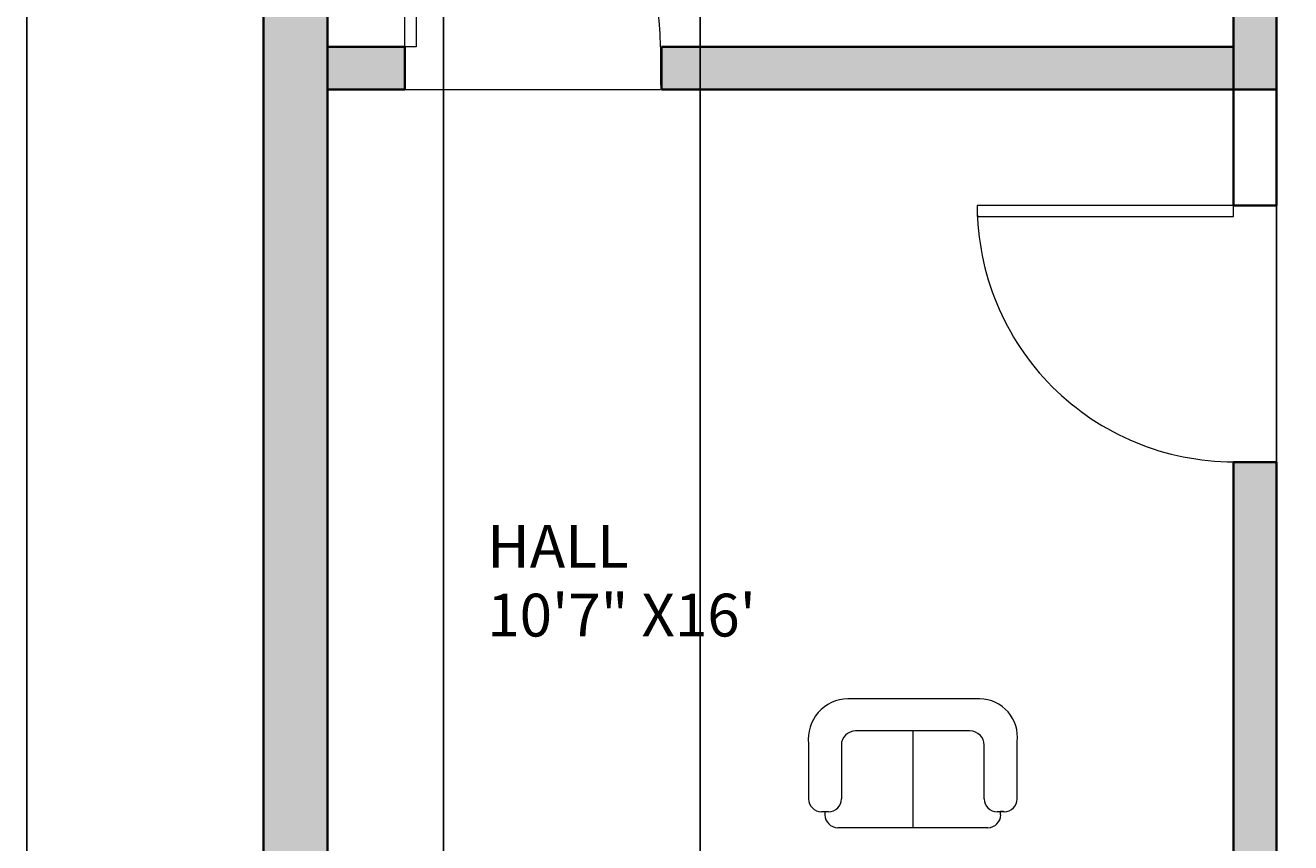
# Model space of a CAD drawing. Units: inches. Extents: x 2070 to 4408, y 1595 to 4269.
# Tile 3 of 20: x 2070 to 2247, y 1835 to 1949. Entities that reach past the tile are written whole.
import ezdxf

# ---------------------------------------------------------------- set-up
doc = ezdxf.new("R2010")
doc.units = ezdxf.units.IN
for name, color, linetype, lineweight in [('A-ANNO-DIMS', 2, 'Continuous', 18), ('A-AREA-IDEN', 7, 'Continuous', 18), ('A-DOOR', 4, 'Continuous', 18), ('A-FURN', 8, 'Continuous', 18), ('A-WALL', 7, 'Continuous', 35)]:
    doc.layers.add(name, color=color, linetype=linetype, lineweight=lineweight)
doc.layers.add('A-WALL-PATT', color=18, linetype='Continuous', lineweight=13, true_color=0x000000)
doc.styles.get("Standard").update_dxf_attribs({"font": 'arial.ttf'})
doc.dimstyles.get("Standard").update_dxf_attribs({"dimtxt": 0.18, "dimasz": 0.18, "dimexe": 0.18, "dimexo": 0.0625, "dimgap": 0.09, "dimtad": 0, "dimtih": 1, "dimtoh": 1, "dimdec": 4, "dimzin": 0, "dimdsep": 46, "dimtxsty": 'Standard', "dimcen": 0.09, "dimadec": 0, "dimazin": 0, "dimtfac": 1, "dimtdec": 4, "dimtofl": 0, "dimtmove": 0, "dimatfit": 3, "dimfxl": 1, "dimtolj": 1, "dimtzin": 0, "dimarcsym": 0})

# ---------------------------------------------------------------- blocks, each defined once
blk = doc.blocks.new('*U4')
for p, q in [((0, 0), (0, -6)), ((40, 0), (40, -6))]:
    blk.add_line(p, q)
blk.add_lwpolyline([(0, 0), (0, 40), (1.75, 40), (1.75, 0)], close=True)
blk.add_arc((0, 0), 40, 0, 90)
blk = doc.blocks.new('*U3')
for p, q in [((0, 0), (0, 6)), ((40, 0), (40, 6))]:
    blk.add_line(p, q)
blk.add_lwpolyline([(0, 0), (0, -40), (1.75, -40), (1.75, 0)], close=True)
blk.add_arc((0, 0), 40, 270, 0)
blk = doc.blocks.new('A$C6D011943')
for p, q in [((1.448, 1.089), (0.332, 1.089)), ((1.364, 0.818), (0.398, 0.818)), ((0.881, 0.818), (0.881, 0)), ((0, 0.709), (0, 0.247)), ((0.278, 0.697), (0.278, 0.244)), ((1.485, 0.244), (1.485, 0.697)), ((1.762, 0.247), (1.762, 0.727)), ((0.109, 0.136), (0.169, 0.136)), ((0.139, 0.109), (0.139, 0.136)), ((1.593, 0.136), (1.654, 0.136)), ((1.648, 0.136), (1.623, 0.136)), ((1.623, 0.109), (1.623, 0.136)), ((1.515, 0), (0.247, 0))]:
    blk.add_line(p, q)
for centre, radius, start, end in [((0.339, 0.748), 0.342, 91.2564, 186.501), ((1.441, 0.766), 0.324, 353.159, 88.6697), ((0.398, 0.697), 0.121, 90, 180), ((1.364, 0.697), 0.121, 0, 90), ((0.109, 0.244), 0.109, 180, 270), ((0.169, 0.244), 0.109, 270, 0), ((1.593, 0.244), 0.109, 180, 270), ((1.654, 0.244), 0.109, 270, 0), ((0.247, 0.109), 0.109, 180, 270), ((1.515, 0.109), 0.109, 270, 0)]:
    blk.add_arc(centre, radius, start, end)
blk = doc.blocks.new('*D24')
at = {"layer": 'A-ANNO-DIMS', "color": 0, "lineweight": -2, "transparency": 16777216}
for p, q in [((2103.13, 2291.4), (2069.84, 2291.4)), ((2070.02, 2291.22), (2070.02, 1960.08)), ((2070.02, 1628.58), (2070.02, 1959.72)), ((2336.13, 1628.4), (2069.84, 1628.4))]:
    blk.add_line(p, q, dxfattribs=at)
at = {"layer": 'A-ANNO-DIMS', "color": 0, "transparency": 16777216}
for points in [[(2069.99, 2291.22), (2070.05, 2291.22), (2070.02, 2291.4)], [(2069.99, 1628.58), (2070.05, 1628.58), (2070.02, 1628.4)]]:
    blk.add_solid(points, dxfattribs=at)
at = {"layer": 'Defpoints', "color": 0, "transparency": 16777216}
for p in [(2070.02, 2291.4), (2103.2, 2291.4), (2336.2, 1628.4)]:
    blk.add_point(p, dxfattribs=at)
at = {"layer": 'A-ANNO-DIMS', "color": 0, "transparency": 16777216, "insert": (2070.02, 1959.9), "char_height": 0.18, "attachment_point": 5}
blk.add_mtext('\\A1;663', dxfattribs=at)
blk = doc.blocks.new('*D29')
at = {"layer": 'A-ANNO-DIMS', "color": 0, "lineweight": -2, "transparency": 16777216}
for p, q in [((2128.44, 2150.34), (2128.44, 1595.04)), ((2164.44, 2150.34), (2164.44, 1595.04)), ((2128.62, 1595.22), (2146.22, 1595.22)), ((2164.26, 1595.22), (2146.65, 1595.22))]:
    blk.add_line(p, q, dxfattribs=at)
at = {"layer": 'A-ANNO-DIMS', "color": 0, "transparency": 16777216}
for points in [[(2128.62, 1595.25), (2128.62, 1595.19), (2128.44, 1595.22)], [(2164.26, 1595.25), (2164.26, 1595.19), (2164.44, 1595.22)]]:
    blk.add_solid(points, dxfattribs=at)
at = {"layer": 'Defpoints', "color": 0, "transparency": 16777216}
for p in [(2128.44, 2150.4), (2164.44, 2150.4), (2164.44, 1595.22)]:
    blk.add_point(p, dxfattribs=at)
at = {"layer": 'A-ANNO-DIMS', "color": 0, "transparency": 16777216, "insert": (2146.44, 1595.22), "char_height": 0.18, "attachment_point": 5}
blk.add_mtext('\\A1;36', dxfattribs=at)
blk = doc.blocks.new('*D32')
at = {"layer": 'A-ANNO-DIMS', "color": 0, "lineweight": -2, "transparency": 16777216}
for p, q in [((2245.2, 2230.58), (2245.2, 1595.04)), ((2340.2, 2230.58), (2340.2, 1595.04)), ((2245.38, 1595.22), (2292.48, 1595.22)), ((2340.02, 1595.22), (2292.92, 1595.22))]:
    blk.add_line(p, q, dxfattribs=at)
at = {"layer": 'A-ANNO-DIMS', "color": 0, "transparency": 16777216}
for points in [[(2245.38, 1595.25), (2245.38, 1595.19), (2245.2, 1595.22)], [(2340.02, 1595.25), (2340.02, 1595.19), (2340.2, 1595.22)]]:
    blk.add_solid(points, dxfattribs=at)
at = {"layer": 'Defpoints', "color": 0, "transparency": 16777216}
for p in [(2245.2, 2230.65), (2340.2, 2230.65), (2340.2, 1595.22)]:
    blk.add_point(p, dxfattribs=at)
at = {"layer": 'A-ANNO-DIMS', "color": 0, "transparency": 16777216, "insert": (2292.7, 1595.22), "char_height": 0.18, "attachment_point": 5}
blk.add_mtext('\\A1;95', dxfattribs=at)

msp = doc.modelspace()

# ---------------------------------------------------------------- hatches: boundary and pattern name
at = {"layer": 'A-WALL-PATT'}
h = msp.add_hatch(color=256, dxfattribs=at)
h.dxf.hatch_style = 1
h.paths.add_polyline_path([(2346.196, 2218.3995), (2346.196, 2282.3995), (2340.196, 2282.3995), (2340.196, 2212.3995), (2345.5866, 2212.3995), (2346.196, 2212.3995)], flags=0)
h.paths.add_polyline_path([(2245.196, 2282.3995), (2239.196, 2282.3995), (2239.196, 2186.3995), (2244.5866, 2186.3995), (2245.196, 2186.3995)], flags=0)
h.paths.add_polyline_path([(2340.196, 2230.6455), (2245.196, 2230.6455), (2245.196, 2224.6455), (2340.196, 2224.6455)], flags=0)
h.paths.add_polyline_path([(2245.196, 2150.3995), (2239.196, 2150.3995), (2164.4362, 2150.3995), (2164.4362, 2144.3995), (2239.196, 2144.3995), (2239.196, 2086.3995), (2239.196, 2067.2711), (2244.5866, 2067.2711), (2245.196, 2067.2711), (2245.196, 2144.3995)], flags=0)
h.paths.add_polyline_path([(2346.196, 2176.3995), (2340.196, 2176.3995), (2340.196, 2086.3995), (2346.196, 2086.3995), (2346.196, 2125.318)], flags=0)
h.paths.add_polyline_path([(2446.196, 2086.3995), (2346.196, 2086.3995), (2340.196, 2086.3995), (2340.196, 2080.3995), (2446.196, 2080.3995)], flags=0)
h.paths.add_polyline_path([(2455.196, 2291.3995), (2103.196, 2291.3995), (2103.196, 1699.3995), (2336.196, 1699.3995), (2336.196, 1628.3995), (2345.196, 1628.3995), (2446.196, 1628.3995), (2454.8846, 1628.3995), (2454.8846, 1699.3995)])
h.paths.add_polyline_path([(2446.196, 2282.3995), (2446.196, 2218.3995), (2446.196, 2212.3995), (2446.196, 2086.3995), (2446.196, 2080.3995), (2446.196, 1708.3995), (2446.196, 1637.3995), (2345.196, 1637.3995), (2345.196, 1699.3995), (2345.196, 1708.3995), (2336.196, 1708.3995), (2112.196, 1708.3995), (2112.196, 2282.3995), (2239.196, 2282.3995), (2245.196, 2282.3995), (2356.196, 2282.3995)], flags=16)
h.paths.add_polyline_path([(2245.196, 2150.3995), (2245.196, 2144.3995), (2245.196, 2067.2711), (2244.5866, 2067.2711), (2239.196, 2067.2711), (2239.196, 2065.6988), (2203.2929, 2065.6988, 0.40145271), (2239.196, 2031.3337), (2244.5866, 2031.3337), (2245.196, 2031.2711), (2245.196, 1924.1525), (2239.196, 1924.1525), (2239.196, 1922.5803), (2203.2929, 1922.5803, 0.40145271), (2239.196, 1888.2151), (2244.5866, 1888.2151), (2245.196, 1888.1525), (2245.196, 1748.3995), (2339.196, 1748.4621, -0.40145271), (2303.2929, 1782.8272), (2303.2585, 1782.8272), (2303.2585, 1784.3995), (2339.196, 1784.3995), (2339.196, 1877.2067), (2291.196, 1877.2067), (2291.196, 1883.2067), (2291.196, 1946.3995), (2291.196, 1952.3995), (2291.196, 2086.3995), (2297.196, 2086.3995), (2302.196, 2086.3995), (2302.196, 2081.0259), (2303.7633, 2081.0259), (2303.7633, 2080.3995), (2338.0148, 2080.3995, 0.00437129), (2338.0203, 2081.0259), (2338.0203, 2086.3995), (2340.196, 2086.3995), (2340.196, 2176.4621), (2345.5866, 2176.4621, 0.40145271), (2381.4896, 2210.8272), (2345.5866, 2210.8272), (2345.5866, 2212.3995), (2340.196, 2212.3995), (2340.196, 2224.6455), (2245.196, 2224.6455), (2245.196, 2186.3995), (2244.5866, 2186.3995), (2239.196, 2186.3995), (2239.196, 2184.8272), (2203.2929, 2184.8272, 0.40145271), (2239.196, 2150.4621), (2244.5866, 2150.4621)], flags=0)
h.paths.add_polyline_path([(2346.196, 2282.3995), (2346.196, 2218.3995), (2377.1813, 2218.3995), (2377.1813, 2212.3995), (2346.196, 2212.3995), (2345.5866, 2212.3995), (2340.196, 2212.3995), (2340.196, 2224.6455), (2245.196, 2224.6455), (2245.196, 2230.6455), (2245.196, 2282.3995), (2292.696, 2256.5225), (2340.196, 2282.3995)], flags=0)
h.paths.add_polyline_path([(2346.196, 2086.3995), (2340.196, 2086.3995), (2340.196, 2080.3995), (2446.196, 2080.3995), (2431.196, 2016.3995), (2446.196, 1952.3995), (2412.196, 1952.3995), (2412.196, 2080.3995), (2340.196, 2080.3995), (2340.196, 2086.3995), (2340.196, 2176.3995), (2346.196, 2176.3995), (2346.196, 2125.318)], flags=0)
h.paths.add_polyline_path([(2186.508, 2270.0471, -0.03755288), (2186.9712, 2269.8581), (2186.9164, 2270.112, -0.02759121)], flags=0)
h.paths.add_polyline_path([(2183.955, 2273.7766, 1), (2188.2945, 2273.7766, 1)], flags=0)
h.paths.add_polyline_path([(2142.5261, 2274.6158, -0.03707541), (2142.5672, 2275.1696), (2142.5672, 2276.826), (2119.8759, 2276.826), (2119.8759, 2263.0962), (2140.4332, 2263.0962), (2142.5672, 2263.0962), (2142.5672, 2274.0621, -0.03707541)], flags=0)
h.paths.add_polyline_path([(2209.8974, 2263.0962), (2209.8974, 2262.2079), (2190.8042, 2262.2079), (2190.8042, 2263.0962)], flags=0)
h.paths.add_polyline_path([(2210.6382, 2276.1833), (2210.6382, 2263.9844), (2190.2185, 2263.9844), (2190.2185, 2276.1833)], flags=0)
h.paths.add_polyline_path([(2188.4362, 2273.7766, -1), (2183.8133, 2273.7766, -1)], flags=0)
h.paths.add_polyline_path([(2245.196, 2150.3995), (2245.196, 2144.3995), (2245.196, 2067.2711), (2239.196, 2067.2711), (2239.196, 2080.3995), (2172.196, 2080.3995), (2172.196, 2000.3995), (2239.196, 2000.3995), (2239.196, 1940.3995), (2159.0187, 1940.3995), (2123.0187, 1940.3995), (2112.196, 1940.3995), (2112.196, 1946.3995), (2123.0187, 1946.3995), (2123.0187, 1982.2238), (2124.586, 1982.2238), (2124.586, 1982.1895, -0.40145271), (2158.8429, 1946.3995), (2159.0187, 1946.3995), (2239.196, 1946.3995), (2239.196, 1994.3995), (2112.196, 1994.3995), (2112.196, 2000.3995), (2139.196, 2040.3995), (2112.196, 2080.3995), (2112.196, 2086.3995), (2239.196, 2086.3995), (2239.196, 2144.3995), (2209.5809, 2144.3995), (2209.5809, 2136.3995), (2203.0809, 2136.3995), (2205.0809, 2130.3996, -0.70257121), (2199.081, 2116.3995, -0.70256205), (2193.0809, 2130.3994), (2195.0809, 2136.3995), (2192.0809, 2136.3995), (2192.0809, 2134.8995), (2189.0809, 2134.8995), (2189.0809, 2135.8995), (2191.0809, 2135.8995), (2191.0809, 2136.3995), (2188.5809, 2136.3995), (2188.5809, 2144.3995), (2164.2481, 2144.3995, -0.39385849), (2130.0035, 2109.5491), (2130.0035, 2109.5147), (2128.4362, 2109.5147), (2128.4362, 2144.3995), (2112.196, 2144.3995), (2112.196, 2150.3995), (2128.4362, 2150.3995), (2128.4362, 2150.7127), (2164.4362, 2150.7127), (2164.4362, 2150.3995), (2239.196, 2150.3995)], flags=0)
h.paths.add_polyline_path([(2188.2075, 2266.8735), (2188.2075, 2211.8632, -0.41421356), (2185.4833, 2209.1391), (2146.7995, 2209.1391, -0.41421356), (2144.0754, 2211.8632), (2144.0754, 2266.8735, -0.41421356), (2146.7995, 2269.5976), (2185.4833, 2269.5976, -0.41421356)], flags=0)
h.paths.add_polyline_path([(2185.0844, 2273.7766, -1), (2187.1651, 2273.7766, -1)], flags=0)
h.paths.add_polyline_path([(2182.0486, 2259.2932), (2168.0953, 2259.2932), (2168.0953, 2260.8424), (2163.7261, 2260.8424), (2163.7261, 2259.2932), (2149.7727, 2259.2932), (2149.7727, 2266.3352), (2163.7261, 2266.3352), (2163.7261, 2261.9839), (2168.0953, 2261.9839), (2168.0953, 2266.3352), (2182.0486, 2266.3352)], flags=0)
h.paths.add_polyline_path([(2148.2585, 2250.2051), (2153.0615, 2241.8861, 0.39807048)], flags=0)
h.paths.add_polyline_path([(2162.7572, 2247.2885), (2153.1461, 2241.7396), (2148.1083, 2250.4653), (2157.7194, 2256.0142)], flags=0)
h.paths.add_polyline_path([(2162.6726, 2247.4351, -0.39286196), (2157.8415, 2255.6313), (2157.6431, 2255.6313), (2157.8696, 2255.7541)], flags=0)
h.paths.add_polyline_path([(2164.2604, 2145.339), (2164.4362, 2144.3995), (2164.4362, 2150.3995), (2164.2604, 2150.7127)], flags=0)
h.paths.add_polyline_path([(2208.5809, 2142.6495), (2208.5809, 2138.3995, -0.41421356), (2207.8309, 2137.3995), (2190.5809, 2137.3995, -0.41421356), (2189.5809, 2138.1495), (2189.5809, 2142.3995, -0.41421356), (2190.3309, 2143.3995), (2207.5809, 2143.3995, -0.41421356)], flags=0)
h.paths.add_polyline_path([(2147.957, 2229.9119), (2154.7494, 2223.1195, 0.39807048)], flags=0)
h.paths.add_polyline_path([(2162.7165, 2230.8473), (2154.8691, 2222.9998), (2147.7446, 2230.1244), (2155.592, 2237.9718)], flags=0)
h.paths.add_polyline_path([(2162.5969, 2230.9669, -0.39807048), (2155.8044, 2237.7594)], flags=0)
h.paths.add_polyline_path([(2391.8776, 2049.9192), (2408.5766, 2049.9192), (2408.5766, 2033.2202), (2408.5766, 1983.123), (2408.5766, 1966.4239), (2391.8776, 1966.4239), (2391.8776, 1983.123), (2341.7804, 1983.123), (2341.7804, 2033.2202), (2391.8776, 2033.2202)], flags=0)
h.paths.add_polyline_path([(2144.1055, 2274.6158, 1), (2148.445, 2274.6158, 1)], flags=0)
h.paths.add_polyline_path([(2148.5867, 2274.6158, -1), (2143.9638, 2274.6158, -1)], flags=0)
h.paths.add_polyline_path([(2145.2349, 2274.6158, -1), (2147.3156, 2274.6158, -1)], flags=0)
edge = h.paths.add_edge_path(flags=0)
edge.add_ellipse((2400.5951, 2040.9436), major_axis=(-4.5109, 0), ratio=0.97544784, start_angle=180, end_angle=270, ccw=False)
edge.add_ellipse((2400.5951, 2040.9436), major_axis=(-4.5109, 0), ratio=0.97544784, start_angle=90, end_angle=180, ccw=False)
edge.add_ellipse((2400.5951, 2040.9436), major_axis=(-4.5109, 0), ratio=0.97544784, start_angle=0, end_angle=90, ccw=False)
edge.add_ellipse((2400.5951, 2040.9436), major_axis=(-4.5109, 0), ratio=0.97544784, start_angle=270, end_angle=360, ccw=False)
h.paths.add_polyline_path([(2199.0809, 2117.3995, -0.73452973), (2195.0809, 2130.3995), (2203.081, 2130.3995, -0.73453329)], flags=0)
h.paths.add_polyline_path([(2141.9147, 2276.0353), (2141.9147, 2263.9844), (2120.4685, 2263.9844), (2120.4685, 2276.0353)], flags=0)
h.paths.add_polyline_path([(2138.4481, 2273.4072), (2138.4481, 2266.7226), (2133.2801, 2266.7226), (2133.2801, 2273.4072)], flags=0)
h.paths.add_polyline_path([(2137.9691, 2272.9175), (2137.9691, 2272.204), (2135.4229, 2272.204), (2135.4229, 2271.6329), (2135.3221, 2270.1051), (2135.3221, 2269.0265), (2135.4229, 2268.6811), (2135.4229, 2267.2011), (2133.7212, 2267.2011), (2133.7212, 2268.6811), (2133.7983, 2269.9587), (2133.7983, 2271.2758), (2133.7212, 2271.6329), (2133.7212, 2273.0065), (2135.717, 2273.0065), (2135.717, 2272.9175)], flags=0)
h.paths.add_polyline_path([(2137.9215, 2271.8264), (2137.9215, 2271.3786), (2137.5182, 2271.3786), (2136.9355, 2271.3786), (2136.3529, 2271.3786), (2135.7703, 2271.3786), (2135.7703, 2271.8264), (2136.1736, 2271.8264), (2136.7562, 2271.8264), (2137.3389, 2271.8264)], flags=0)
h.paths.add_polyline_path([(2137.9215, 2271.692), (2137.5182, 2271.692), (2136.9355, 2271.513), (2137.3389, 2271.513)], flags=0)
h.paths.add_polyline_path([(2136.3529, 2271.692), (2135.7703, 2271.513), (2136.1736, 2271.513), (2136.7562, 2271.692)], flags=0)
h.paths.add_polyline_path([(2137.9215, 2271.513), (2137.5182, 2271.513), (2136.7562, 2271.747), (2136.7562, 2271.692), (2137.3389, 2271.692)], flags=0)
h.paths.add_polyline_path([(2137.8207, 2270.4664), (2137.8207, 2270.0971), (2137.8207, 2269.627), (2137.8207, 2269.1569), (2137.8207, 2268.6868), (2137.3837, 2268.6868), (2136.6442, 2268.6868), (2135.9271, 2268.6868), (2135.9271, 2269.0562), (2135.9271, 2269.5263), (2135.9271, 2269.9963), (2135.9271, 2270.4664), (2136.3641, 2270.4664), (2137.0812, 2270.4664)], flags=0)
h.paths.add_polyline_path([(2137.3837, 2269.627), (2137.8207, 2269.627), (2137.8207, 2269.5263), (2137.3837, 2269.5263), (2137.3837, 2269.1569), (2137.8207, 2269.1569), (2137.3837, 2269.0562), (2137.3837, 2268.6868), (2137.0812, 2268.6868), (2137.0812, 2269.0562), (2136.6442, 2269.0562), (2136.6442, 2268.6868), (2136.3641, 2268.6868), (2136.3641, 2269.0562), (2135.9271, 2269.0562), (2135.9271, 2269.1569), (2136.3641, 2269.1569), (2136.3641, 2269.5263), (2135.9271, 2269.5263), (2135.9271, 2269.627), (2136.3641, 2269.627), (2136.3641, 2269.9963), (2135.9271, 2269.9963), (2136.3641, 2270.0971), (2136.3641, 2270.4664), (2136.6442, 2270.4664), (2136.6442, 2270.0971), (2137.0812, 2270.0971), (2137.0812, 2270.4664), (2137.3837, 2270.4664), (2137.3837, 2270.0971), (2137.8207, 2270.0971), (2137.3837, 2269.9963)], flags=0)
h.paths.add_polyline_path([(2137.5182, 2271.8264), (2137.5182, 2271.692), (2137.3389, 2271.3786), (2137.3389, 2271.513)], flags=0)
h.paths.add_polyline_path([(2137.8179, 2267.8138), (2137.8179, 2267.6879), (2137.1876, 2267.6879), (2136.4733, 2267.6879), (2135.759, 2267.6879), (2135.759, 2267.8138), (2136.3893, 2267.8138), (2137.1036, 2267.8138)], flags=0)
h.paths.add_polyline_path([(2137.0812, 2269.9963), (2137.0812, 2269.627), (2137.0812, 2269.1569), (2136.6442, 2269.1569), (2136.6442, 2269.5263), (2136.6442, 2269.9963)], flags=0)
h.paths.add_polyline_path([(2136.3529, 2271.8264), (2136.3529, 2271.692), (2136.1736, 2271.3786), (2136.1736, 2271.513)], flags=0)
h.paths.add_polyline_path([(2136.4733, 2267.8138), (2136.4733, 2267.6879), (2136.3893, 2267.6879), (2136.3893, 2267.8138)], flags=0)
h.paths.add_polyline_path([(2407.9087, 2032.5522), (2407.9087, 1983.7909), (2359.81, 1983.7909, -0.00912788), (2359.0575, 1983.7909), (2342.4483, 1983.7909), (2342.4483, 2032.5522)], flags=0)
h.paths.add_polyline_path([(2389.1838, 2023.1358), (2353.7856, 2023.1358), (2353.7856, 1985.4867, -0.09210376), (2350.2788, 1988.655), (2350.2788, 2026.6426), (2389.1838, 2026.6426)], flags=0)
h.paths.add_polyline_path([(2352.6166, 2024.3048), (2351.4477, 2024.3048), (2351.4477, 2025.4737), (2352.6166, 2025.4737)], flags=0)
h.paths.add_polyline_path([(2399.6319, 2026.7589), (2404.3661, 2026.7589, -0.41421356), (2407.0379, 2024.087), (2407.0379, 2013.4908, -0.41421356), (2404.3661, 2010.819), (2399.6319, 2010.819, -0.41421356), (2396.96, 2013.4908), (2396.96, 2024.087, -0.41421356)], flags=0)
h.paths.add_polyline_path([(2399.6319, 2026.0909), (2404.3661, 2026.0909, -0.41421356), (2406.37, 2024.087), (2406.37, 2013.4908, -0.41421356), (2404.3661, 2011.487), (2399.6319, 2011.487, -0.41421356), (2397.628, 2013.4908), (2397.628, 2024.087, -0.41421356)], flags=0)
h.paths.add_polyline_path([(2399.6319, 2002.3217), (2404.3661, 2002.3217, -0.41421356), (2407.0379, 1999.6498), (2407.0379, 1989.0536, -0.41421356), (2404.3661, 1986.3818), (2399.6319, 1986.3818, -0.41421356), (2396.96, 1989.0536), (2396.96, 1999.6498, -0.41421356)], flags=0)
h.paths.add_polyline_path([(2399.6319, 2001.6537), (2404.3661, 2001.6537, -0.41421356), (2406.37, 1999.6498), (2406.37, 1989.0536, -0.41421356), (2404.3661, 1987.0497), (2399.6319, 1987.0497, -0.41421356), (2397.628, 1989.0536), (2397.628, 1999.6498, -0.41421356)], flags=0)
edge = h.paths.add_edge_path(flags=0)
edge.add_ellipse((2400.5951, 1975.3996), major_axis=(-4.5109, 0), ratio=0.97544784, start_angle=-180, end_angle=-90, ccw=False)
edge.add_ellipse((2400.5951, 1975.3996), major_axis=(-4.5109, 0), ratio=0.97544784, start_angle=90, end_angle=180, ccw=False)
edge.add_ellipse((2400.5951, 1975.3996), major_axis=(-4.5109, 0), ratio=0.97544784, start_angle=0, end_angle=90, ccw=False)
edge.add_ellipse((2400.5951, 1975.3996), major_axis=(-4.5109, 0), ratio=0.97544784, start_angle=-90, end_angle=0, ccw=False)
h.paths.add_polyline_path([(2345.196, 1910.3995), (2366.4386, 1910.3995), (2366.4386, 1925.4555), (2392.3856, 1925.4555), (2392.3856, 1933.5025), (2400.1399, 1925.4555), (2392.3856, 1919.8795), (2392.3856, 1925.4555), (2366.4386, 1925.4555), (2366.4386, 1910.3995), (2381.196, 1910.3995), (2405.196, 1910.3995), (2405.196, 1898.3995), (2446.196, 1898.3995), (2446.196, 1886.3995), (2405.196, 1886.3995), (2405.196, 1874.3995), (2446.196, 1874.3995), (2446.196, 1862.3995), (2405.196, 1862.3995), (2405.196, 1850.3995), (2446.196, 1850.3995), (2446.196, 1838.3995), (2405.196, 1838.3995), (2405.196, 1826.3995), (2446.196, 1826.3995), (2446.196, 1814.3995), (2405.196, 1814.3995), (2405.196, 1802.3995), (2446.196, 1802.3995), (2446.196, 1798.3995), (2446.196, 1792.3995), (2405.196, 1792.3995), (2405.196, 1910.3995), (2381.196, 1910.3995), (2381.196, 1792.3995), (2345.196, 1792.3995)], flags=0)
h.paths.add_polyline_path([(2333.0944, 1863.3993, -0.41421356), (2334.7225, 1861.7712), (2334.7225, 1859.329), (2335.2653, 1859.329, -0.41421356), (2337.4361, 1857.1582), (2337.4361, 1843.862, -0.41421356), (2335.2653, 1841.6911, -0.41421356), (2337.4361, 1839.5203), (2337.4361, 1827.5808, -0.41421356), (2335.2653, 1825.41, -0.41421356), (2337.4361, 1823.2392), (2337.4361, 1808.5862, -0.41421356), (2335.2653, 1806.4153), (2334.7225, 1806.4153), (2334.7225, 1803.9732, -0.41421356), (2333.0944, 1802.3451), (2317.356, 1802.3451), (2317.0846, 1802.3451, -0.41421356), (2315.7279, 1803.7018), (2315.7279, 1803.8646), (2313.8284, 1803.8646, -0.41421356), (2311.6576, 1806.0354), (2311.6576, 1823.2015, -0.39597602), (2313.6834, 1825.3765, -0.43384798), (2311.6576, 1827.2718), (2311.6576, 1839.761, -0.41421356), (2313.5571, 1841.6604), (2313.8284, 1841.6604), (2333.8159, 1841.6604, -0.04213623), (2334.1798, 1841.6911, -0.41421356), (2332.009, 1843.862), (2332.009, 1857.1582, -0.41421356), (2334.1798, 1859.329), (2317.356, 1859.329), (2317.0846, 1859.329, -0.41421356), (2315.7279, 1860.6858), (2315.7279, 1862.0426, -0.41421356), (2317.0846, 1863.3993), (2317.356, 1863.3993)], flags=0)
h.paths.add_polyline_path([(2208.8475, 1848.9818), (2208.8475, 1840.9741, -0.41421356), (2207.0458, 1839.1724), (2206.5453, 1839.1721), (2206.5453, 1838.7218, -0.40985861), (2204.7704, 1836.9203), (2183.7501, 1836.9203, -0.41858196), (2181.9216, 1838.7218), (2181.9216, 1839.1721), (2181.421, 1839.1724, -0.41421356), (2179.6193, 1840.9741), (2179.6193, 1848.6817, -0.44064415), (2185.1126, 1854.9874), (2203.3852, 1854.9874, -0.45707961)], flags=0)
h.paths.add_polyline_path([(2204.243, 1848.4815), (2204.243, 1848.4815, 0.41725335), (2202.2204, 1850.4833), (2186.2049, 1850.4833, 0.4111805), (2184.2237, 1848.4815), (2184.2237, 1848.4815, -0.4111807), (2186.2049, 1850.4833), (2202.2204, 1850.4833, -0.41725315)], flags=0)
h.paths.add_polyline_path([(2234.7177, 1830.228), (2234.7176, 1781.6047, -0.41421356), (2233.4381, 1780.3252), (2218.6064, 1780.3252, -0.41421356), (2217.8387, 1781.0929), (2217.8387, 1783.3961, -0.41421356), (2218.6064, 1784.1639), (2218.6065, 1796.9595, -0.41421356), (2219.886, 1798.239, -0.41421356), (2218.6065, 1799.5186), (2218.6065, 1812.3142, -0.41421356), (2219.8861, 1813.5938, -0.41421356), (2218.6065, 1814.8733), (2218.6065, 1827.6689, -0.41421356), (2217.8388, 1828.4367), (2217.8388, 1830.7399, -0.41421356), (2218.6065, 1831.5076), (2233.4382, 1831.5076, -0.41421356)], flags=0)
h.paths.add_polyline_path([(2230.6344, 1827.6689, -0.41421356), (2231.4021, 1826.9012), (2231.4021, 1784.9316, -0.41421356), (2230.6343, 1784.1639), (2221.1853, 1784.1639), (2221.1853, 1827.6689)], flags=0)
h.paths.add_polyline_path([(2222.7208, 1798.239), (2221.6971, 1798.239), (2221.6971, 1813.5938), (2222.7208, 1813.5938)], flags=0)
h.paths.add_polyline_path([(2206.5453, 1773.935), (2206.5453, 1773.4848), (2206.9457, 1773.4848), (2207.0458, 1773.4845, -0.41421356), (2208.8475, 1771.6827), (2208.8475, 1763.675, -0.44222432), (2203.6505, 1757.6695), (2185.3851, 1757.6695, -0.45508402), (2179.6193, 1763.9752), (2179.6193, 1771.6827, -0.41421356), (2181.421, 1773.4845), (2181.421, 1773.4848), (2181.9216, 1773.4848), (2181.9216, 1773.935, -0.40985861), (2183.6965, 1775.7366), (2204.7167, 1775.7366, -0.41858196)], flags=0)
h.paths.add_polyline_path([(2202.2619, 1762.1736), (2186.2464, 1762.1736, -0.41725315), (2184.2237, 1764.1754), (2184.2237, 1764.1754, 0.41725335), (2186.2464, 1762.1736), (2202.2619, 1762.1736, 0.4111805), (2204.243, 1764.1754), (2204.243, 1764.1754, -0.4111807)], flags=0)
h.paths.add_polyline_path([(2313.0034, 1713.1906), (2312.997, 1713.1697), (2313.0123, 1713.1612)], flags=0)
h.paths.add_polyline_path([(2305.7314, 1721.0488), (2305.6257, 1721.1994), (2305.4853, 1721.084)], flags=0)
h.paths.add_polyline_path([(2307.5562, 1726.1427), (2307.6186, 1726.1026), (2307.5737, 1726.0477), (2308.5692, 1720.6434), (2310.5345, 1721.2985), (2310.5721, 1721.411), (2310.6958, 1721.3523), (2313.8453, 1722.4021), (2314.9351, 1723.8033), (2314.9294, 1723.9165), (2315.0028, 1723.8903), (2313.874, 1722.4389), (2313.8697, 1722.4102), (2308.5692, 1720.6434), (2308.9864, 1720.122), (2309.0665, 1720.0971), (2309.053, 1720.0387), (2310.9235, 1717.7005), (2311.4182, 1717.6259), (2311.2918, 1717.2402), (2312.0655, 1716.2731), (2312.1081, 1716.2606), (2312.0969, 1716.2339), (2308.5692, 1720.6434), (2305.2249, 1717.745), (2305.232, 1717.704), (2305.1665, 1717.6944), (2308.5692, 1720.6434)], flags=0)
h.paths.add_polyline_path([(2288.2072, 1714.3431), (2288.2008, 1714.3222), (2288.216, 1714.3137)], flags=0)
h.paths.add_polyline_path([(2280.9352, 1722.2013), (2280.8295, 1722.3519), (2280.689, 1722.2365)], flags=0)
h.paths.add_polyline_path([(2282.76, 1727.2952), (2282.8224, 1727.2551), (2282.7775, 1727.2002), (2283.773, 1721.7959), (2285.7383, 1722.451), (2285.7759, 1722.5635), (2285.8995, 1722.5048), (2289.0491, 1723.5546), (2290.1389, 1724.9558), (2290.1332, 1725.069), (2290.2065, 1725.0428), (2289.0777, 1723.5915), (2289.0735, 1723.5628), (2283.773, 1721.7959), (2284.1901, 1721.2745), (2284.2703, 1721.2496), (2284.2567, 1721.1913), (2286.1273, 1718.8531), (2286.622, 1718.7785), (2286.4956, 1718.3927), (2287.2692, 1717.4256), (2287.3119, 1717.4131), (2287.3006, 1717.3864), (2283.773, 1721.7959), (2280.4286, 1718.8975), (2280.4357, 1718.8565), (2280.3703, 1718.8469), (2283.773, 1721.7959)], flags=0)
h.paths.add_polyline_path([(2302.0672, 1721.8694), (2301.8205, 1721.8572), (2301.7578, 1722.1787), (2299.415, 1724.5215), (2299.103, 1724.4694), (2299.0662, 1724.8703)], flags=0)
h.paths.add_polyline_path([(2264.5643, 1715.4956), (2264.5579, 1715.4747), (2264.5731, 1715.4662)], flags=0)
h.paths.add_polyline_path([(2257.2923, 1723.3538), (2257.1865, 1723.5044), (2257.0461, 1723.389)], flags=0)
h.paths.add_polyline_path([(2259.117, 1728.4477), (2259.1795, 1728.4077), (2259.1345, 1728.3527), (2260.13, 1722.9484), (2262.0954, 1723.6036), (2262.133, 1723.716), (2262.2566, 1723.6573), (2265.4061, 1724.7071), (2266.4959, 1726.1083), (2266.4902, 1726.2215), (2266.5636, 1726.1953), (2265.4348, 1724.744), (2265.4305, 1724.7153), (2260.13, 1722.9484), (2260.5472, 1722.427), (2260.6273, 1722.4022), (2260.6138, 1722.3438), (2262.4843, 1720.0056), (2262.979, 1719.931), (2262.8526, 1719.5452), (2263.6263, 1718.5781), (2263.6689, 1718.5656), (2263.6577, 1718.5389), (2260.13, 1722.9484), (2256.7857, 1720.05), (2256.7928, 1720.009), (2256.7273, 1719.9994), (2260.13, 1722.9484)], flags=0)
h.paths.add_polyline_path([(2277.2709, 1723.0219), (2277.0243, 1723.0097), (2276.9616, 1723.3312), (2274.6187, 1725.6741), (2274.3067, 1725.6219), (2274.27, 1726.0228)], flags=0)
h.paths.add_polyline_path([(2253.628, 1724.1744), (2253.3814, 1724.1622), (2253.3186, 1724.4838), (2250.9758, 1726.8266), (2250.6638, 1726.7744), (2250.627, 1727.1753)], flags=0)
h.paths.add_polyline_path([(2161.9194, 1715.4956), (2161.913, 1715.4747), (2161.9282, 1715.4662)], flags=0)
h.paths.add_polyline_path([(2154.6474, 1723.3538), (2154.5416, 1723.5044), (2154.4012, 1723.389)], flags=0)
h.paths.add_polyline_path([(2162.7899, 1724.744), (2162.7856, 1724.7153), (2157.4851, 1722.9484), (2157.9023, 1722.427), (2157.9824, 1722.4022), (2157.9689, 1722.3438), (2159.8394, 1720.0056), (2160.3341, 1719.931), (2160.2078, 1719.5452), (2160.9814, 1718.5781), (2161.024, 1718.5656), (2161.0128, 1718.5389), (2157.4851, 1722.9484), (2154.1408, 1720.05), (2154.1479, 1720.009), (2154.0824, 1719.9994), (2157.4851, 1722.9484), (2156.4721, 1728.4477), (2156.5346, 1728.4077), (2156.4896, 1728.3527), (2157.4851, 1722.9484), (2159.4505, 1723.6036), (2159.4881, 1723.716), (2159.6117, 1723.6573), (2162.7612, 1724.7071), (2163.851, 1726.1083), (2163.8453, 1726.2215), (2163.9187, 1726.1953)], flags=0)
h.paths.add_polyline_path([(2150.9831, 1724.1744), (2150.7365, 1724.1622), (2150.6738, 1724.4838), (2148.3309, 1726.8266), (2148.0189, 1726.7744), (2147.9822, 1727.1753)], flags=0)
h.paths.add_polyline_path([(2132.5099, 1716.6482), (2132.5035, 1716.6272), (2132.5187, 1716.6187)], flags=0)
h.paths.add_polyline_path([(2125.2379, 1724.5064), (2125.1322, 1724.6569), (2124.9917, 1724.5415)], flags=0)
h.paths.add_polyline_path([(2133.3804, 1725.8965), (2133.3762, 1725.8678), (2128.0757, 1724.101), (2128.4928, 1723.5795), (2128.5729, 1723.5547), (2128.5594, 1723.4963), (2130.43, 1721.1581), (2130.9246, 1721.0835), (2130.7983, 1720.6977), (2131.5719, 1719.7306), (2131.6146, 1719.7181), (2131.6033, 1719.6914), (2128.0757, 1724.101), (2124.7313, 1721.2025), (2124.7384, 1721.1615), (2124.6729, 1721.1519), (2128.0757, 1724.101), (2127.0626, 1729.6002), (2127.1251, 1729.5602), (2127.0801, 1729.5052), (2128.0757, 1724.101), (2130.041, 1724.7561), (2130.0786, 1724.8685), (2130.2022, 1724.8098), (2133.3517, 1725.8597), (2134.4415, 1727.2608), (2134.4358, 1727.3741), (2134.5092, 1727.3478)], flags=0)
h.paths.add_polyline_path([(2121.5736, 1725.3269), (2121.327, 1725.3148), (2121.2643, 1725.6363), (2118.9214, 1727.9791), (2118.6094, 1727.9269), (2118.5727, 1728.3279)], flags=0)
h.paths.add_polyline_path([(2433.3904, 1646.406), (2433.384, 1646.3851), (2433.3992, 1646.3766)], flags=0)
h.paths.add_polyline_path([(2426.1184, 1654.2642), (2426.0127, 1654.4148), (2425.8722, 1654.2994)], flags=0)
h.paths.add_polyline_path([(2427.9432, 1659.3581), (2428.0056, 1659.318), (2427.9606, 1659.2631), (2428.9562, 1653.8588), (2430.9215, 1654.514), (2430.9591, 1654.6264), (2431.0827, 1654.5677), (2434.2323, 1655.6175), (2435.322, 1657.0187), (2435.3163, 1657.1319), (2435.3897, 1657.1057), (2434.2609, 1655.6544), (2434.2567, 1655.6257), (2428.9562, 1653.8588), (2429.3733, 1653.3374), (2429.4534, 1653.3126), (2429.4399, 1653.2542), (2431.3105, 1650.916), (2431.8051, 1650.8414), (2431.6788, 1650.4556), (2432.4524, 1649.4885), (2432.4951, 1649.476), (2432.4838, 1649.4493), (2428.9562, 1653.8588), (2425.6118, 1650.9604), (2425.6189, 1650.9194), (2425.5535, 1650.9098), (2428.9562, 1653.8588)], flags=0)
h.paths.add_polyline_path([(2376.63, 1645.4912), (2376.6236, 1645.4703), (2376.6388, 1645.4617)], flags=0)
h.paths.add_polyline_path([(2369.358, 1653.3494), (2369.2523, 1653.5), (2369.1118, 1653.3845)], flags=0)
h.paths.add_polyline_path([(2371.1828, 1658.4432), (2371.2452, 1658.4032), (2371.2003, 1658.3482), (2372.1958, 1652.944), (2374.1611, 1653.5991), (2374.1987, 1653.7116), (2374.3224, 1653.6528), (2377.4719, 1654.7027), (2378.5617, 1656.1038), (2378.556, 1656.2171), (2378.6293, 1656.1908), (2377.5005, 1654.7395), (2377.4963, 1654.7108), (2372.1958, 1652.944), (2372.6129, 1652.4225), (2372.6931, 1652.3977), (2372.6795, 1652.3393), (2374.5501, 1650.0011), (2375.0448, 1649.9265), (2374.9184, 1649.5407), (2375.692, 1648.5737), (2375.7347, 1648.5611), (2375.7234, 1648.5344), (2372.1958, 1652.944), (2368.8514, 1650.0456), (2368.8586, 1650.0046), (2368.7931, 1649.995), (2372.1958, 1652.944)], flags=0)
h.paths.add_polyline_path([(2404.0947, 1645.0338), (2404.0883, 1645.0128), (2404.1035, 1645.0043)], flags=0)
h.paths.add_polyline_path([(2396.8227, 1652.892), (2396.717, 1653.0425), (2396.5765, 1652.9271)], flags=0)
h.paths.add_polyline_path([(2398.6475, 1657.9858), (2398.7099, 1657.9458), (2398.665, 1657.8908), (2399.6605, 1652.4866), (2401.6258, 1653.1417), (2401.6634, 1653.2541), (2401.7871, 1653.1954), (2404.9366, 1654.2453), (2406.0264, 1655.6464), (2406.0207, 1655.7596), (2406.094, 1655.7334), (2404.9652, 1654.2821), (2404.961, 1654.2534), (2399.6605, 1652.4866), (2400.0776, 1651.9651), (2400.1578, 1651.9403), (2400.1442, 1651.8819), (2402.0148, 1649.5437), (2402.5095, 1649.4691), (2402.3831, 1649.0833), (2403.1567, 1648.1162), (2403.1994, 1648.1037), (2403.1881, 1648.077), (2399.6605, 1652.4866), (2396.3162, 1649.5881), (2396.3233, 1649.5471), (2396.2578, 1649.5375), (2399.6605, 1652.4866)], flags=0)
h.paths.add_polyline_path([(2419.4532, 1658.0857), (2422.4541, 1655.0848), (2422.2075, 1655.0726), (2422.1448, 1655.3941), (2419.8019, 1657.737), (2419.4899, 1657.6848)], flags=0)
h.paths.add_polyline_path([(2390.1575, 1656.7135), (2393.1584, 1653.7125), (2392.9118, 1653.7004), (2392.8491, 1654.0219), (2390.5063, 1656.3647), (2390.1943, 1656.3125)], flags=0)
h.paths.add_polyline_path([(2362.6928, 1657.1709), (2365.6937, 1654.1699), (2365.4471, 1654.1578), (2365.3844, 1654.4793), (2363.0416, 1656.8221), (2362.7295, 1656.77)], flags=0)
h.paths.add_polyline_path([(2419.9523, 2037.8601), (2440.2872, 2037.8601), (2440.2872, 2047.1732), (2419.9523, 2047.1732)], flags=8)
h.paths.add_polyline_path([(2370.186, 1698.9005), (2413.6287, 1698.9005), (2413.6287, 1708.0908), (2370.186, 1708.0908)], flags=8)
h.paths.add_polyline_path([(2370.1656, 1708.5185), (2430.0857, 1708.5185), (2430.0857, 1717.8316), (2370.1656, 1717.8316)], flags=8)
h.paths.add_polyline_path([(2254.1469, 1788.1883), (2302.2471, 1788.1883), (2302.2471, 1797.3786), (2254.1469, 1797.3786)], flags=8)
h.paths.add_polyline_path([(2254.1264, 1797.8063), (2326.1448, 1797.8063), (2326.1448, 1807.1194), (2254.1264, 1807.1194)], flags=8)
h.paths.add_polyline_path([(2300.08, 1914.5069), (2338.861, 1914.5069), (2338.861, 1923.6972), (2300.08, 1923.6972)], flags=8)
h.paths.add_polyline_path([(2300.0595, 1924.1249), (2331.5882, 1924.1249), (2331.5882, 1933.438), (2300.0595, 1933.438)], flags=8)
h.paths.add_polyline_path([(2176.6905, 1716.4567), (2224.1441, 1716.4567), (2224.1441, 1725.647), (2176.6905, 1725.647)], flags=8)
h.paths.add_polyline_path([(2176.67, 1726.0747), (2245.9176, 1726.0747), (2245.9176, 1735.3878), (2176.67, 1735.3878)], flags=8)
h.paths.add_polyline_path([(2339.997, 2039.7696), (2388.1034, 2039.7696), (2388.1034, 2048.9661), (2339.997, 2048.9661)], flags=8)
h.paths.add_polyline_path([(2339.9776, 2049.3928), (2388.7204, 2049.3928), (2388.7204, 2058.7059), (2339.9776, 2058.7059)], flags=8)
h.paths.add_polyline_path([(2366.0063, 2161.3825), (2409.449, 2161.3825), (2409.449, 2170.5728), (2366.0063, 2170.5728)], flags=8)
h.paths.add_polyline_path([(2365.9868, 2171.0016), (2405.879, 2171.0016), (2405.879, 2180.3085), (2365.9868, 2180.3085)], flags=8)
h.paths.add_polyline_path([(2366.0102, 2247.0726), (2407.12, 2247.0726), (2407.12, 2256.263), (2366.0102, 2256.263)], flags=8)
h.paths.add_polyline_path([(2365.9897, 2256.6906), (2397.9686, 2256.6906), (2397.9686, 2266.0037), (2365.9897, 2266.0037)], flags=8)
h.paths.add_polyline_path([(2271.8465, 2102.7885), (2307.6541, 2102.7885), (2307.6541, 2111.9849), (2271.8465, 2111.9849)], flags=8)
h.paths.add_polyline_path([(2271.8281, 2112.4126), (2304.2673, 2112.4126), (2304.2673, 2121.7196), (2271.8281, 2121.7196)], flags=8)
h.paths.add_polyline_path([(2141.6408, 2187.5934), (2182.108, 2187.5934), (2182.108, 2196.7837), (2141.6408, 2196.7837)], flags=8)
h.paths.add_polyline_path([(2141.6203, 2197.2114), (2190.3631, 2197.2114), (2190.3631, 2206.5245), (2141.6203, 2206.5245)], flags=8)
h.paths.add_polyline_path([(2165.7271, 2103.039), (2211.5027, 2103.039), (2211.5027, 2112.2293), (2165.7271, 2112.2293)], flags=8)
h.paths.add_polyline_path([(2165.7077, 2112.658), (2185.1033, 2112.658), (2185.1033, 2121.965), (2165.7077, 2121.965)], flags=8)
h.paths.add_polyline_path([(2174.945, 2048.0789), (2211.3973, 2048.0789), (2211.3973, 2057.2693), (2174.945, 2057.2693)], flags=8)
h.paths.add_polyline_path([(2174.9256, 2057.698), (2194.3212, 2057.698), (2194.3212, 2067.0049), (2174.9256, 2067.0049)], flags=8)
h.paths.add_polyline_path([(2164.8305, 1965.8394), (2202.9649, 1965.8394), (2202.9649, 1975.0297), (2164.8305, 1975.0297)], flags=8)
h.paths.add_polyline_path([(2164.8111, 1975.4584), (2184.2067, 1975.4584), (2184.2067, 1984.7654), (2164.8111, 1984.7654)], flags=8)
h.paths.add_polyline_path([(2133.0392, 1862.086), (2173.5065, 1862.086), (2173.5065, 1871.2763), (2133.0392, 1871.2763)], flags=8)
h.paths.add_polyline_path([(2133.0709, 1871.8585), (2157.0382, 1871.8585), (2157.0382, 1880.8585), (2133.0709, 1880.8585)], flags=8)
h.paths.add_polyline_path([(2406.4423, 1923.5541), (2418.8209, 1923.5541), (2418.8209, 1932.7199), (2406.4423, 1932.7199)], flags=8)
h = msp.add_hatch(color=256, dxfattribs=at)
h.dxf.hatch_style = 1
h.paths.add_polyline_path([(2245.196, 2282.3995), (2239.196, 2282.3995), (2239.196, 2186.3995), (2244.5866, 2186.3995), (2245.196, 2186.3995)])
h.paths.add_polyline_path([(2340.196, 2230.6455), (2245.196, 2230.6455), (2245.196, 2224.6455), (2340.196, 2224.6455)])
h.paths.add_polyline_path([(2346.196, 2282.3995), (2340.196, 2282.3995), (2340.196, 2212.3995), (2345.5866, 2212.3995), (2346.196, 2212.3995), (2346.196, 2218.3995)])
h.paths.add_polyline_path([(2245.196, 2144.3995), (2245.196, 2150.3995), (2239.196, 2150.3995), (2164.4362, 2150.3995), (2164.4362, 2144.3995), (2239.196, 2144.3995), (2239.196, 2086.3995), (2239.196, 2067.2711), (2244.5866, 2067.2711), (2245.196, 2067.2711)])
h.paths.add_polyline_path([(2128.4362, 2150.3995), (2112.196, 2150.3995), (2112.196, 2144.3995), (2128.4362, 2144.3995), (2128.4362, 2145.339)])
h.paths.add_polyline_path([(2239.196, 2086.3995), (2112.196, 2086.3995), (2112.196, 2080.3995), (2239.196, 2080.3995)])
h.paths.add_polyline_path([(2172.196, 2080.3995), (2166.196, 2080.3995), (2166.196, 2000.3995), (2172.196, 2000.3995)])
h.paths.add_polyline_path([(2239.196, 2000.3995), (2112.196, 2000.3995), (2112.196, 1994.3995), (2239.196, 1994.3995)])
h.paths.add_polyline_path([(2245.196, 2031.2711), (2239.196, 2031.2711), (2239.196, 2000.3995), (2239.196, 1940.3995), (2245.196, 1940.3995)])
h.paths.add_polyline_path([(2239.196, 1946.3995), (2159.0187, 1946.3995), (2159.0187, 1940.3995), (2239.196, 1940.3995)])
h.paths.add_polyline_path([(2123.0187, 1946.3995), (2112.196, 1946.3995), (2112.196, 1940.3995), (2123.0187, 1940.3995)])
h.paths.add_polyline_path([(2377.1813, 2218.3995), (2346.196, 2218.3995), (2346.196, 2212.3995), (2377.1813, 2212.3995)])
h.paths.add_polyline_path([(2446.196, 2218.3995), (2413.1813, 2218.3995), (2413.1813, 2212.3995), (2446.196, 2212.3995)])
h.paths.add_polyline_path([(2446.196, 2086.3995), (2346.196, 2086.3995), (2340.196, 2086.3995), (2340.196, 2080.3995), (2446.196, 2080.3995)], flags=17)
h.paths.add_polyline_path([(2346.196, 2125.318), (2346.196, 2176.3995), (2340.196, 2176.3995), (2340.196, 2086.3995), (2346.196, 2086.3995)])
h.paths.add_polyline_path([(2245.196, 1888.1525), (2239.196, 1888.1525), (2239.196, 1748.3995), (2245.196, 1748.3995)])
h.paths.add_polyline_path([(2345.196, 1748.3995), (2239.196, 1748.3995), (2112.196, 1748.3995), (2112.196, 1742.3995), (2239.196, 1742.3995), (2345.196, 1742.3995)])
h.paths.add_polyline_path([(2297.196, 2080.3995), (2297.196, 2086.3995), (2291.196, 2086.3995), (2291.196, 1952.3995), (2291.196, 1946.3995), (2339.196, 1946.3995), (2339.196, 1883.2067), (2291.196, 1883.2067), (2291.196, 1877.2067), (2339.196, 1877.2067), (2339.196, 1784.3995), (2345.196, 1784.3995), (2345.196, 1792.3995), (2345.196, 1946.3995), (2446.196, 1946.3995), (2446.196, 1952.3995), (2297.196, 1952.3995)])

# ---------------------------------------------------------------- linework, layer by layer
at = {"layer": 'A-DOOR'}
msp.add_line((2123.0187, 1940.3995), (2158.8429, 1940.3995), dxfattribs=at)
at = {"layer": 'A-WALL'}
for p, q in [((2239.196, 1924.1525), (2239.196, 2031.2711)), ((2245.196, 2031.2711), (2245.196, 1924.1525)), ((2239.196, 1994.3995), (2239.196, 1946.3995)), ((2112.196, 1946.3995), (2112.196, 1940.3995)), ((2123.0187, 1946.3995), (2112.196, 1946.3995)), ((2123.0187, 1940.3995), (2123.0187, 1946.3995)), ((2239.196, 1946.3995), (2159.0187, 1946.3995)), ((2159.0187, 1946.3995), (2159.0187, 1940.3995)), ((2112.196, 1940.3995), (2123.0187, 1940.3995)), ((2112.196, 1940.3995), (2123.0187, 1940.3995)), ((2159.0187, 1940.3995), (2239.196, 1940.3995)), ((2239.196, 1940.3995), (2239.196, 1924.1525)), ((2239.196, 1940.3995), (2245.196, 1940.3995)), ((2245.196, 1940.3995), (2245.196, 1924.1525)), ((2245.196, 1924.1525), (2239.196, 1924.1525)), ((2239.196, 1888.1525), (2245.196, 1888.1525)), ((2239.196, 1888.1525), (2239.196, 1748.3995)), ((2239.196, 1748.3995), (2239.196, 1888.1525)), ((2245.196, 1888.1525), (2245.196, 1748.3995))]:
    msp.add_line(p, q, dxfattribs=at)
for points in [[(2336.196, 1699.3995), (2103.196, 1699.3995), (2103.196, 2291.3995), (2455.196, 2291.3995), (2455.196, 1699.3995), (2454.8846, 1699.3995)], [(2336.196, 1708.3995), (2112.196, 1708.3995), (2112.196, 2282.3995), (2446.196, 2282.3995), (2446.196, 2218.3995)]]:
    msp.add_lwpolyline(points, dxfattribs=at)

# ---------------------------------------------------------------- block references
at = {"layer": 'A-DOOR', "xscale": 0.8956071672485885, "yscale": 0.8956071672485885, "zscale": 0.8956071672485885}
msp.add_blockref('*U4', (2123.0187, 1946.3995), dxfattribs=at)
at = {"layer": 'A-DOOR', "xscale": 0.8984361948159364, "yscale": 0.8984361948159364, "zscale": 0.8984361948159364, "rotation": 270}
msp.add_blockref('*U3', (2239.196, 1924.1525), dxfattribs=at)
at = {"layer": 'A-FURN', "xscale": 16.58622898764873, "yscale": 16.58622898764873, "zscale": 16.58622898764873}
msp.add_blockref('A$C6D011943', (2179.6193, 1836.9201), dxfattribs=at)

# ---------------------------------------------------------------- texts
at = {"layer": 'A-AREA-IDEN'}
for s, p in [('HALL', (2134.5709, 1873.3585)), ('10\'7" X16\'', (2134.5709, 1863.72))]:
    msp.add_text(s, height=6, dxfattribs=at).set_placement(p)

# ---------------------------------------------------------------- dimensions: what is measured, and where the dimension line sits
at = {"layer": 'A-ANNO-DIMS'}
dim = msp.add_linear_dim(base=(2070.016, 2291.3995), p1=(2336.196, 1628.3995), p2=(2103.196, 2291.3995), angle=90, dimstyle='Standard', override={"dimdec": 0, "dimlfac": 1, "dimrnd": 0, "dimzin": 0, "dimdsep": 46, "dimlunit": 2}, dxfattribs=at)
dim.commit()
dim.dimension.update_dxf_attribs({"geometry": '*D24', "text_midpoint": (2070.016, 1959.8995)})
for base, p1, p2, picture, middle in [((2340.196, 1595.2195), (2245.196, 2230.6455), (2340.196, 2230.6455), '*D32', (2292.696, 1595.2195)), ((2164.4362, 1595.2195), (2128.4362, 2150.3995), (2164.4362, 2150.3995), '*D29', (2146.4362, 1595.2195))]:
    dim = msp.add_linear_dim(base=base, p1=p1, p2=p2, dimstyle='Standard', override={"dimdec": 0, "dimlfac": 1, "dimrnd": 0, "dimzin": 0, "dimdsep": 46, "dimlunit": 2}, dxfattribs=at)
    dim.commit()
    dim.dimension.update_dxf_attribs({"geometry": picture, "text_midpoint": middle})

doc.saveas('drawing.dxf')
